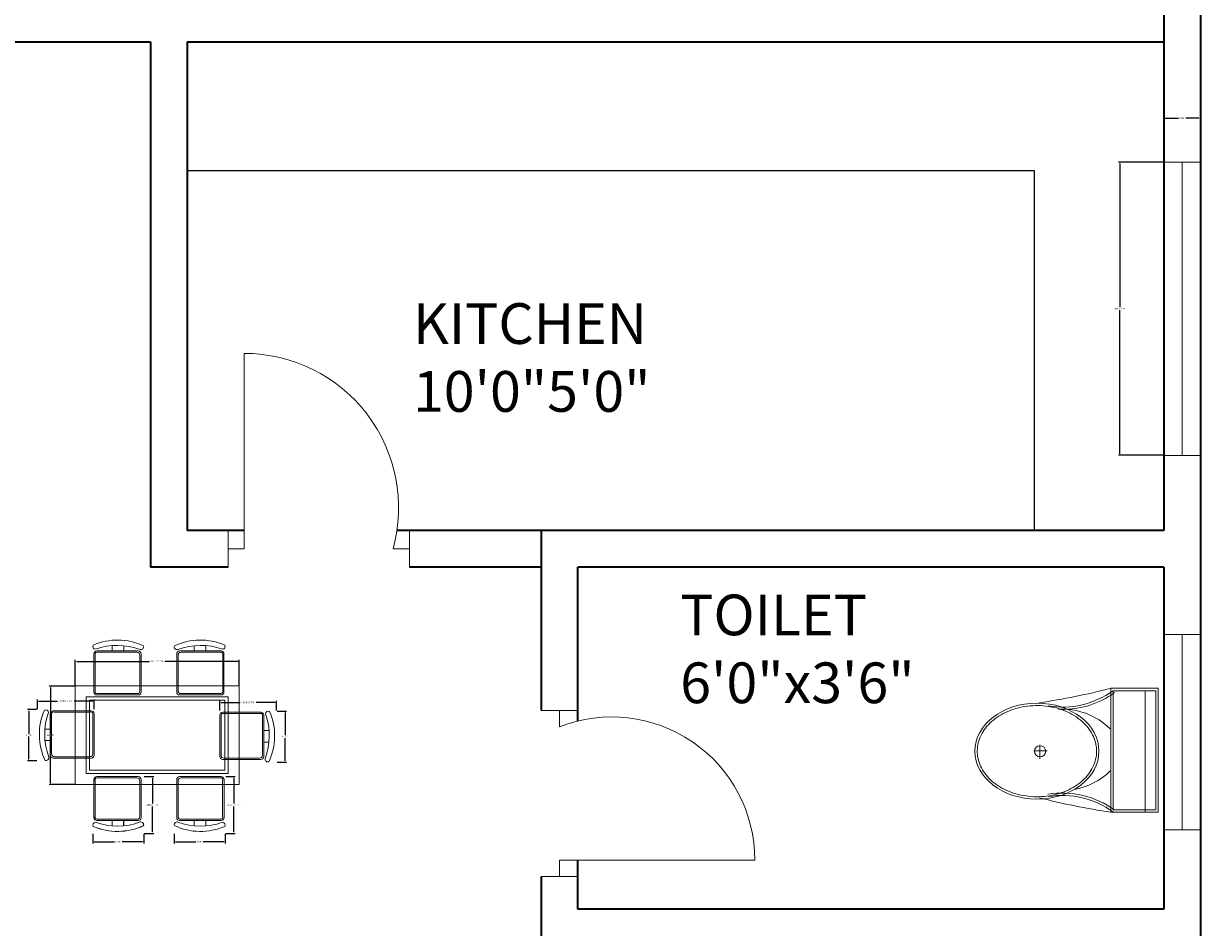
# Model space of a CAD drawing. Units: inches. Extents: x 2234 to 3001, y 1541 to 2386.
# Tile 9 of 12: x 2744 to 2888, y 1891 to 2002. Entities that reach past the tile are written whole.
import ezdxf

# ---------------------------------------------------------------- set-up
doc = ezdxf.new("R2010")
doc.units = ezdxf.units.IN
for name, color, linetype, lineweight in [('A-ANNO-DIMS', 2, 'Continuous', 18), ('A-AREA-IDEN', 7, 'Continuous', 18), ('A-DOOR', 3, 'Continuous', 18), ('A-FLOR-CASE', 8, 'Continuous', 25), ('A-FLOR-FIXT', 9, 'Continuous', 18), ('A-FURN', 9, 'Continuous', 13), ('A-GLAZ', 4, 'Continuous', 18), ('A-WALL', 7, 'Continuous', 35)]:
    doc.layers.add(name, color=color, linetype=linetype, lineweight=lineweight)
doc.styles.get("Standard").update_dxf_attribs({"font": 'arial.ttf'})
doc.dimstyles.get("Standard").update_dxf_attribs({"dimtxt": 0.18, "dimasz": 0.18, "dimexe": 0.18, "dimexo": 0.0625, "dimgap": 0.09, "dimtad": 0, "dimtih": 1, "dimtoh": 1, "dimdec": 4, "dimzin": 0, "dimdsep": 46, "dimtxsty": 'Standard', "dimcen": 0.09, "dimadec": 0, "dimazin": 0, "dimtfac": 1, "dimtdec": 4, "dimtofl": 0, "dimtmove": 0, "dimatfit": 3, "dimfxl": 1, "dimtolj": 1, "dimtzin": 0, "dimarcsym": 0})

# ---------------------------------------------------------------- blocks, each defined once
blk = doc.blocks.new('A$C31115884')
for p, q in [((283.1, 497.7), (223.4, 497.7)), ((257.5, 466.4), (257.5, 523.2)), ((0, 200), (0, 0)), ((520, 200), (0, 200)), ((520, 0), (520, 200)), ((10, 190), (10, 10)), ((510, 190), (10, 190)), ((510, 10), (510, 190)), ((510, 54.5), (0, 54.5)), ((10, 10), (510, 10)), ((0, 0), (520, 0))]:
    blk.add_line(p, q)
blk.add_circle((255.6, 496.4), 23.6)
for centre, radius, start, end in [((2777.7, -204.6), 2807, 165.4549, 171.7133), ((3237, 905), 2807, 188.2867, 194.5451), ((-294.5, 403.3), 364.7, 324.2091, 9.3499), ((-294.5, 403.3), 374.7, 324.2091, 9.3499), ((805.8, 403.3), 364.7, 170.6501, 215.7909), ((139.5, 406.2), 293.5, 315.8436, 2.6563), ((805.8, 403.3), 374.7, 179.2036, 215.7909), ((383.6, 406.2), 293.5, 190.2774, 224.1564)]:
    blk.add_arc(centre, radius, start, end)
blk.add_ellipse((256.2, 509.9), major_axis=(0, -260.7), ratio=0.772727)
blk.add_open_spline([(256.2, 259.2), (263.1, 259.2), (270, 259.7), (287.8, 262.3), (298.7, 265.1), (319.9, 273.1), (330.2, 278.4), (350.1, 291.1), (359.7, 298.7), (377.7, 315.9), (386.2, 325.5), (401.7, 346.6), (408.8, 358.1), (421.3, 382.5), (426.8, 395.5), (435.9, 422.4), (439.5, 436.4), (444.8, 465.1), (446.5, 479.7), (447.9, 509.2), (447.6, 524), (445, 553.3), (442.7, 567.8), (436.3, 596), (432.1, 609.7), (421.9, 636), (416, 648.6), (402.5, 672.1), (395, 683), (378.6, 703), (369.8, 712.1), (351.1, 728), (341.3, 734.8), (320.9, 746.2), (310.4, 750.7), (288.9, 757.3), (278, 759.4), (256, 761), (245, 760.6), (223.1, 757.2), (212.3, 754.3), (191.1, 746.1), (180.8, 740.7), (160.9, 727.8), (151.4, 720.1), (133.5, 702.7), (125.1, 693), (109.6, 671.7), (102.6, 660.2), (90.2, 635.7), (84.9, 622.7), (76, 595.6), (72.4, 581.6), (67.2, 552.9), (65.6, 538.2), (64.4, 508.8), (64.8, 494), (67.5, 464.7), (69.9, 450.2), (76.6, 422), (80.8, 408.3), (91.1, 382.2), (97.2, 369.7), (110.8, 346.3), (118.4, 335.4), (134.8, 315.6), (143.7, 306.7), (162.4, 290.9), (172.3, 284.2), (192.8, 273), (203.3, 268.6), (224.8, 262.2), (235.8, 260.2), (249.9, 259.3), (253, 259.2), (256.2, 259.2)], degree=3, knots=[0, 0, 0, 0, 0.110105, 0.110105, 0.285049, 0.285049, 0.459994, 0.459994, 0.634938, 0.634938, 0.809882, 0.809882, 0.984827, 0.984827, 1.159771, 1.159771, 1.334715, 1.334715, 1.50966, 1.50966, 1.684604, 1.684604, 1.859549, 1.859549, 2.034493, 2.034493, 2.209437, 2.209437, 2.384382, 2.384382, 2.559326, 2.559326, 2.73427, 2.73427, 2.909215, 2.909215, 3.084159, 3.084159, 3.259103, 3.259103, 3.434048, 3.434048, 3.608992, 3.608992, 3.783936, 3.783936, 3.958881, 3.958881, 4.133825, 4.133825, 4.30877, 4.30877, 4.483714, 4.483714, 4.658658, 4.658658, 4.833603, 4.833603, 5.008547, 5.008547, 5.183491, 5.183491, 5.358436, 5.358436, 5.53338, 5.53338, 5.708324, 5.708324, 5.883269, 5.883269, 6.058213, 6.058213, 6.233158, 6.233158, 6.283185, 6.283185, 6.283185, 6.283185])
blk = doc.blocks.new('TABLE-DINING-RECT')
for points in [[(0, 12.09), (20.14, 12.09), (20.14, 0), (0, 0)], [(0, 12.09), (20.14, 12.09), (20.14, 0), (0, 0)], [(1.34, 10.74), (18.8, 10.74), (18.8, 1.34), (1.34, 1.34)], [(1.34, 10.74), (18.8, 10.74), (18.8, 1.34), (1.34, 1.34)], [(1.75, 10.34), (18.4, 10.34), (18.4, 1.75), (1.75, 1.75)], [(1.75, 10.34), (18.4, 10.34), (18.4, 1.75), (1.75, 1.75)]]:
    blk.add_lwpolyline(points, close=True)
blk = doc.blocks.new('CHAIR-DINING-A')
for points in [[(5.76, 1.34, 0.414214), (6.12, 1.7), (6.12, 6.38, 0.414214), (5.76, 6.74), (0.67, 6.74, 0.414214), (0.31, 6.38), (0.31, 1.7, 0.414214), (0.67, 1.34), (5.76, 1.34)], [(5.76, 1.34, 0.414214), (6.12, 1.7), (6.12, 6.38, 0.414214), (5.76, 6.74), (0.67, 6.74, 0.414214), (0.31, 6.38), (0.31, 1.7, 0.414214), (0.67, 1.34), (5.76, 1.34)], [(5.92, 1.12, -0.175809), (0.43, 1.16, 0.578392), (0.02, 0.71, 0.214524), (6.21, 0.62, 0.552014), (5.92, 1.12, -0.065079)], [(5.92, 1.12, -0.175809), (0.43, 1.16, 0.578392), (0.02, 0.71, 0.214524), (6.21, 0.62, 0.552014), (5.92, 1.12, -0.065079)], [(2.45, 1.34), (2.45, 0.7, -0.064759)], [(2.45, 1.34), (2.45, 0.7, -0.064759)]]:
    blk.add_lwpolyline(points, format="xyb")
blk.add_lwpolyline([(5.76, 1.5), (0.83, 1.5, -0.414214), (0.47, 1.86), (0.47, 6.22, -0.414214), (0.83, 6.58), (5.76, 6.58, -0.512069), (5.95, 6.22), (5.95, 1.86, -0.512069)], format="xyb", close=True)
blk.add_lwpolyline([(5.76, 1.5), (0.83, 1.5, -0.414214), (0.47, 1.86), (0.47, 6.22, -0.414214), (0.83, 6.58), (5.76, 6.58, -0.512069), (5.95, 6.22), (5.95, 1.86, -0.512069)], format="xyb", close=True)
blk.add_lwpolyline([(3.88, 0.69), (3.88, 1.34)])
blk.add_lwpolyline([(3.88, 0.69), (3.88, 1.34)])
blk = doc.blocks.new('CHAIR-DINING-B')
for points in [[(5.76, 1.34, 0.414214), (6.12, 1.7), (6.12, 6.38, 0.414214), (5.76, 6.74), (0.67, 6.74, 0.414214), (0.31, 6.38), (0.31, 1.7, 0.414214), (0.67, 1.34), (5.76, 1.34)], [(5.76, 1.34, 0.414214), (6.12, 1.7), (6.12, 6.38, 0.414214), (5.76, 6.74), (0.67, 6.74, 0.414214), (0.31, 6.38), (0.31, 1.7, 0.414214), (0.67, 1.34), (5.76, 1.34)], [(5.92, 1.12, -0.175809), (0.43, 1.16, 0.578392), (0.02, 0.71, 0.214524), (6.21, 0.62, 0.552014), (5.92, 1.12, -0.065079)], [(5.92, 1.12, -0.175809), (0.43, 1.16, 0.578392), (0.02, 0.71, 0.214524), (6.21, 0.62, 0.552014), (5.92, 1.12, -0.065079)], [(2.45, 1.34), (2.45, 0.7, -0.064759)], [(2.45, 1.34), (2.45, 0.7, -0.064759)]]:
    blk.add_lwpolyline(points, format="xyb")
blk.add_lwpolyline([(5.76, 1.5), (0.83, 1.5, -0.414214), (0.47, 1.86), (0.47, 6.22, -0.414214), (0.83, 6.58), (5.76, 6.58, -0.512069), (5.95, 6.22), (5.95, 1.86, -0.512069)], format="xyb", close=True)
blk.add_lwpolyline([(5.76, 1.5), (0.83, 1.5, -0.414214), (0.47, 1.86), (0.47, 6.22, -0.414214), (0.83, 6.58), (5.76, 6.58, -0.512069), (5.95, 6.22), (5.95, 1.86, -0.512069)], format="xyb", close=True)
blk.add_lwpolyline([(3.88, 0.69), (3.88, 1.34)])
blk.add_lwpolyline([(3.88, 0.69), (3.88, 1.34)])
blk = doc.blocks.new('CHAIR-DINING-C')
for points in [[(1.16, 0.43, -0.578392), (0.71, 0.02, -0.214524), (0.62, 6.21, -0.552014), (1.12, 5.92, 0.175809), (1.16, 0.43)], [(1.34, 5.76, -0.414214), (1.7, 6.11), (6.38, 6.11, -0.414214), (6.74, 5.76), (6.74, 0.66, -0.414214), (6.38, 0.31), (1.7, 0.31, -0.414214), (1.34, 0.66), (1.34, 5.76)], [(1.34, 2.45), (0.7, 2.45, 0.064759)]]:
    blk.add_lwpolyline(points, format="xyb")
blk.add_lwpolyline([(1.5, 5.76), (1.5, 0.83, 0.414214), (1.86, 0.47), (6.22, 0.47, 0.414214), (6.58, 0.83), (6.58, 5.76, 0.512069), (6.22, 5.95), (1.86, 5.95, 0.512069)], format="xyb", close=True)
blk.add_lwpolyline([(0.69, 3.88), (1.34, 3.88)])
blk = doc.blocks.new('CHAIR-DINING-F')
for points in [[(5.58, 1.34), (0.49, 1.34, -0.414214), (0.13, 1.7), (0.13, 6.38, -0.414214), (0.49, 6.74), (5.58, 6.74, -0.414214), (5.94, 6.38), (5.94, 1.7, -0.414214), (5.58, 1.34)], [(5.82, 1.16, -0.578392), (6.23, 0.71, -0.214524), (0.04, 0.62, -0.552014), (0.33, 1.12, 0.175809), (5.82, 1.16)], [(3.79, 1.34), (3.79, 0.7, 0.064759)]]:
    blk.add_lwpolyline(points, format="xyb")
blk.add_lwpolyline([(0.49, 1.5), (5.42, 1.5, 0.414214), (5.78, 1.86), (5.78, 6.22, 0.414214), (5.42, 6.58), (0.49, 6.58, 0.512069), (0.29, 6.22), (0.29, 1.86, 0.512069)], format="xyb", close=True)
blk.add_lwpolyline([(2.37, 0.69), (2.37, 1.34)])
blk = doc.blocks.new('WIN-24-A')
for p, q in [((0, 24), (4.5, 24)), ((4.5, 24), (2.25, 24)), ((2.25, 24), (2.25, 0)), ((2.25, 0), (0, 0)), ((0, 0), (4.5, 0))]:
    blk.add_line(p, q)
blk = doc.blocks.new('WIN-36')
for p, q in [((0, 36), (4.5, 36)), ((4.5, 36), (2.25, 36)), ((2.25, 36), (2.25, 0)), ((2.25, 0), (0, 0)), ((0, 0), (4.5, 0))]:
    blk.add_line(p, q)
blk = doc.blocks.new('*D33')
at = {"layer": 'A-ANNO-DIMS', "color": 0, "lineweight": -2, "transparency": 16777216}
for p, q in [((2883.69, 1985.34), (2878.17, 1985.34)), ((2878.35, 1985.16), (2878.35, 1967.52)), ((2878.35, 1949.52), (2878.35, 1967.15)), ((2883.69, 1949.34), (2878.17, 1949.34))]:
    blk.add_line(p, q, dxfattribs=at)
at = {"layer": 'A-ANNO-DIMS', "color": 0, "transparency": 16777216}
for points in [[(2878.32, 1985.16), (2878.38, 1985.16), (2878.35, 1985.34)], [(2878.32, 1949.52), (2878.38, 1949.52), (2878.35, 1949.34)]]:
    blk.add_solid(points, dxfattribs=at)
at = {"layer": 'Defpoints', "color": 0, "transparency": 16777216}
for p in [(2883.75, 1985.34), (2878.35, 1949.34), (2883.75, 1949.34)]:
    blk.add_point(p, dxfattribs=at)
at = {"layer": 'A-ANNO-DIMS', "color": 0, "transparency": 16777216, "insert": (2878.35, 1967.34), "char_height": 0.18, "attachment_point": 5}
blk.add_mtext('\\A1;WIN 36 TYP.', dxfattribs=at)
blk = doc.blocks.new('*D34')
at = {"layer": 'A-ANNO-DIMS', "color": 0, "lineweight": -2, "transparency": 16777216}
for p, q in [((2883.75, 1985.4), (2883.75, 1990.92)), ((2883.93, 1990.74), (2885.55, 1990.74)), ((2888.07, 1990.74), (2886.46, 1990.74)), ((2888.25, 1985.4), (2888.25, 1990.92))]:
    blk.add_line(p, q, dxfattribs=at)
at = {"layer": 'A-ANNO-DIMS', "color": 0, "transparency": 16777216}
for points in [[(2883.93, 1990.77), (2883.93, 1990.71), (2883.75, 1990.74)], [(2888.07, 1990.77), (2888.07, 1990.71), (2888.25, 1990.74)]]:
    blk.add_solid(points, dxfattribs=at)
at = {"layer": 'Defpoints', "color": 0, "transparency": 16777216}
for p in [(2883.75, 1990.74), (2883.75, 1985.34), (2888.25, 1985.34)]:
    blk.add_point(p, dxfattribs=at)
at = {"layer": 'A-ANNO-DIMS', "color": 0, "transparency": 16777216, "insert": (2886, 1990.74), "char_height": 0.18, "attachment_point": 5}
blk.add_mtext('\\A1;5 TYP.', dxfattribs=at)
blk = doc.blocks.new('*D39')
at = {"layer": 'A-ANNO-DIMS', "color": 0, "lineweight": -2, "transparency": 16777216}
for p, q in [((2749.99, 1921.07), (2749.99, 1924.21)), ((2750.17, 1924.03), (2759.1, 1924.03)), ((2769.95, 1924.03), (2761.02, 1924.03)), ((2770.13, 1921.07), (2770.13, 1924.21))]:
    blk.add_line(p, q, dxfattribs=at)
at = {"layer": 'A-ANNO-DIMS', "color": 0, "transparency": 16777216}
for points in [[(2750.17, 1924.06), (2750.17, 1924), (2749.99, 1924.03)], [(2769.95, 1924.06), (2769.95, 1924), (2770.13, 1924.03)]]:
    blk.add_solid(points, dxfattribs=at)
at = {"layer": 'Defpoints', "color": 0, "transparency": 16777216}
for p in [(2770.13, 1924.03), (2749.99, 1921.01), (2770.13, 1921.01)]:
    blk.add_point(p, dxfattribs=at)
at = {"layer": 'A-ANNO-DIMS', "color": 0, "transparency": 16777216, "insert": (2760.06, 1924.03), "char_height": 0.18, "attachment_point": 5}
blk.add_mtext('\\A1;TABLE 20 TYP.', dxfattribs=at)
blk = doc.blocks.new('*D40')
at = {"layer": 'A-ANNO-DIMS', "color": 0, "lineweight": -2, "transparency": 16777216}
for p, q in [((2749.93, 1921.01), (2746.79, 1921.01)), ((2746.97, 1920.83), (2746.97, 1915.15)), ((2746.97, 1909.1), (2746.97, 1914.79)), ((2749.93, 1908.92), (2746.79, 1908.92))]:
    blk.add_line(p, q, dxfattribs=at)
at = {"layer": 'A-ANNO-DIMS', "color": 0, "transparency": 16777216}
for points in [[(2746.94, 1920.83), (2747, 1920.83), (2746.97, 1921.01)], [(2746.94, 1909.1), (2747, 1909.1), (2746.97, 1908.92)]]:
    blk.add_solid(points, dxfattribs=at)
at = {"layer": 'Defpoints', "color": 0, "transparency": 16777216}
for p in [(2746.97, 1921.01), (2749.99, 1921.01), (2749.99, 1908.92)]:
    blk.add_point(p, dxfattribs=at)
at = {"layer": 'A-ANNO-DIMS', "color": 0, "transparency": 16777216, "insert": (2746.97, 1914.97), "char_height": 0.18, "attachment_point": 5}
blk.add_mtext('\\A1;12 TYP.', dxfattribs=at)
blk = doc.blocks.new('*D41')
at = {"layer": 'A-ANNO-DIMS', "color": 0, "lineweight": -2, "transparency": 16777216}
for p, q in [((2767.75, 1918), (2767.75, 1919.17)), ((2774.73, 1918), (2774.73, 1919.17)), ((2767.93, 1918.99), (2770.24, 1918.99)), ((2774.55, 1918.99), (2772.24, 1918.99))]:
    blk.add_line(p, q, dxfattribs=at)
at = {"layer": 'A-ANNO-DIMS', "color": 0, "transparency": 16777216}
for points in [[(2767.93, 1919.02), (2767.93, 1918.96), (2767.75, 1918.99)], [(2774.55, 1919.02), (2774.55, 1918.96), (2774.73, 1918.99)]]:
    blk.add_solid(points, dxfattribs=at)
at = {"layer": 'Defpoints', "color": 0, "transparency": 16777216}
for p in [(2767.75, 1918.99), (2767.75, 1917.94), (2774.73, 1917.94)]:
    blk.add_point(p, dxfattribs=at)
at = {"layer": 'A-ANNO-DIMS', "color": 0, "transparency": 16777216, "insert": (2771.24, 1918.99), "char_height": 0.18, "attachment_point": 5}
blk.add_mtext('\\A1;CHAIR A 7 TYP.', dxfattribs=at)
blk = doc.blocks.new('*D42')
at = {"layer": 'A-ANNO-DIMS', "color": 0, "lineweight": -2, "transparency": 16777216}
for p, q in [((2774.79, 1917.94), (2775.95, 1917.94)), ((2775.77, 1917.76), (2775.77, 1914.98)), ((2775.77, 1911.83), (2775.77, 1914.61)), ((2774.79, 1911.65), (2775.95, 1911.65))]:
    blk.add_line(p, q, dxfattribs=at)
at = {"layer": 'A-ANNO-DIMS', "color": 0, "transparency": 16777216}
for points in [[(2775.74, 1917.76), (2775.8, 1917.76), (2775.77, 1917.94)], [(2775.74, 1911.83), (2775.8, 1911.83), (2775.77, 1911.65)]]:
    blk.add_solid(points, dxfattribs=at)
at = {"layer": 'Defpoints', "color": 0, "transparency": 16777216}
for p in [(2774.73, 1917.94), (2775.77, 1917.94), (2774.73, 1911.65)]:
    blk.add_point(p, dxfattribs=at)
at = {"layer": 'A-ANNO-DIMS', "color": 0, "transparency": 16777216, "insert": (2775.77, 1914.8), "char_height": 0.18, "attachment_point": 5}
blk.add_mtext('\\A1;6 TYP.', dxfattribs=at)
blk = doc.blocks.new('*D43')
at = {"layer": 'A-ANNO-DIMS', "color": 0, "lineweight": -2, "transparency": 16777216}
for p, q in [((2768.48, 1909.89), (2769.64, 1909.89)), ((2769.46, 1909.71), (2769.46, 1906.58)), ((2769.46, 1903.09), (2769.46, 1906.22)), ((2768.48, 1902.91), (2769.64, 1902.91))]:
    blk.add_line(p, q, dxfattribs=at)
at = {"layer": 'A-ANNO-DIMS', "color": 0, "transparency": 16777216}
for points in [[(2769.43, 1909.71), (2769.49, 1909.71), (2769.46, 1909.89)], [(2769.43, 1903.09), (2769.49, 1903.09), (2769.46, 1902.91)]]:
    blk.add_solid(points, dxfattribs=at)
at = {"layer": 'Defpoints', "color": 0, "transparency": 16777216}
for p in [(2768.42, 1909.89), (2769.46, 1909.89), (2768.42, 1902.91)]:
    blk.add_point(p, dxfattribs=at)
at = {"layer": 'A-ANNO-DIMS', "color": 0, "transparency": 16777216, "insert": (2769.46, 1906.4), "char_height": 0.18, "attachment_point": 5}
blk.add_mtext('\\A1;CHAIR B 7 TYP.', dxfattribs=at)
blk = doc.blocks.new('*D44')
at = {"layer": 'A-ANNO-DIMS', "color": 0, "lineweight": -2, "transparency": 16777216}
for p, q in [((2762.13, 1902.85), (2762.13, 1901.69)), ((2762.31, 1901.87), (2764.82, 1901.87)), ((2768.24, 1901.87), (2765.73, 1901.87)), ((2768.42, 1902.85), (2768.42, 1901.69))]:
    blk.add_line(p, q, dxfattribs=at)
at = {"layer": 'A-ANNO-DIMS', "color": 0, "transparency": 16777216}
for points in [[(2762.31, 1901.9), (2762.31, 1901.84), (2762.13, 1901.87)], [(2768.24, 1901.9), (2768.24, 1901.84), (2768.42, 1901.87)]]:
    blk.add_solid(points, dxfattribs=at)
at = {"layer": 'Defpoints', "color": 0, "transparency": 16777216}
for p in [(2762.13, 1902.91), (2768.42, 1902.91), (2768.42, 1901.87)]:
    blk.add_point(p, dxfattribs=at)
at = {"layer": 'A-ANNO-DIMS', "color": 0, "transparency": 16777216, "insert": (2765.27, 1901.87), "char_height": 0.18, "attachment_point": 5}
blk.add_mtext('\\A1;6 TYP.', dxfattribs=at)
blk = doc.blocks.new('*D45')
at = {"layer": 'A-ANNO-DIMS', "color": 0, "lineweight": -2, "transparency": 16777216}
for p, q in [((2745.34, 1918.18), (2745.34, 1919.34)), ((2745.52, 1919.16), (2747.82, 1919.16)), ((2752.14, 1919.16), (2749.84, 1919.16)), ((2752.32, 1918.18), (2752.32, 1919.34))]:
    blk.add_line(p, q, dxfattribs=at)
at = {"layer": 'A-ANNO-DIMS', "color": 0, "transparency": 16777216}
for points in [[(2745.52, 1919.19), (2745.52, 1919.13), (2745.34, 1919.16)], [(2752.14, 1919.19), (2752.14, 1919.13), (2752.32, 1919.16)]]:
    blk.add_solid(points, dxfattribs=at)
at = {"layer": 'Defpoints', "color": 0, "transparency": 16777216}
for p in [(2752.32, 1919.16), (2745.34, 1918.11), (2752.32, 1918.11)]:
    blk.add_point(p, dxfattribs=at)
at = {"layer": 'A-ANNO-DIMS', "color": 0, "transparency": 16777216, "insert": (2748.83, 1919.16), "char_height": 0.18, "attachment_point": 5}
blk.add_mtext('\\A1;CHAIR C 7 TYP.', dxfattribs=at)
blk = doc.blocks.new('*D46')
at = {"layer": 'A-ANNO-DIMS', "color": 0, "lineweight": -2, "transparency": 16777216}
for p, q in [((2745.28, 1918.11), (2744.12, 1918.11)), ((2744.3, 1917.93), (2744.3, 1915.15)), ((2744.3, 1912.01), (2744.3, 1914.79)), ((2745.28, 1911.83), (2744.12, 1911.83))]:
    blk.add_line(p, q, dxfattribs=at)
at = {"layer": 'A-ANNO-DIMS', "color": 0, "transparency": 16777216}
for points in [[(2744.27, 1917.93), (2744.33, 1917.93), (2744.3, 1918.11)], [(2744.27, 1912.01), (2744.33, 1912.01), (2744.3, 1911.83)]]:
    blk.add_solid(points, dxfattribs=at)
at = {"layer": 'Defpoints', "color": 0, "transparency": 16777216}
for p in [(2744.3, 1918.11), (2745.34, 1918.11), (2745.34, 1911.83)]:
    blk.add_point(p, dxfattribs=at)
at = {"layer": 'A-ANNO-DIMS', "color": 0, "transparency": 16777216, "insert": (2744.3, 1914.97), "char_height": 0.18, "attachment_point": 5}
blk.add_mtext('\\A1;6 TYP.', dxfattribs=at)
blk = doc.blocks.new('*D51')
at = {"layer": 'A-ANNO-DIMS', "color": 0, "lineweight": -2, "transparency": 16777216}
for p, q in [((2758.48, 1909.89), (2759.65, 1909.89)), ((2759.47, 1909.71), (2759.47, 1906.58)), ((2759.47, 1903.09), (2759.47, 1906.22)), ((2758.48, 1902.91), (2759.65, 1902.91))]:
    blk.add_line(p, q, dxfattribs=at)
at = {"layer": 'A-ANNO-DIMS', "color": 0, "transparency": 16777216}
for points in [[(2759.44, 1909.71), (2759.5, 1909.71), (2759.47, 1909.89)], [(2759.44, 1903.09), (2759.5, 1903.09), (2759.47, 1902.91)]]:
    blk.add_solid(points, dxfattribs=at)
at = {"layer": 'Defpoints', "color": 0, "transparency": 16777216}
for p in [(2758.42, 1909.89), (2759.47, 1909.89), (2758.42, 1902.91)]:
    blk.add_point(p, dxfattribs=at)
at = {"layer": 'A-ANNO-DIMS', "color": 0, "transparency": 16777216, "insert": (2759.47, 1906.4), "char_height": 0.18, "attachment_point": 5}
blk.add_mtext('\\A1;CHAIR F 7 TYP.', dxfattribs=at)
blk = doc.blocks.new('*D52')
at = {"layer": 'A-ANNO-DIMS', "color": 0, "lineweight": -2, "transparency": 16777216}
for p, q in [((2752.14, 1902.85), (2752.14, 1901.69)), ((2752.32, 1901.87), (2754.82, 1901.87)), ((2758.24, 1901.87), (2755.74, 1901.87)), ((2758.42, 1902.85), (2758.42, 1901.69))]:
    blk.add_line(p, q, dxfattribs=at)
at = {"layer": 'A-ANNO-DIMS', "color": 0, "transparency": 16777216}
for points in [[(2752.32, 1901.9), (2752.32, 1901.84), (2752.14, 1901.87)], [(2758.24, 1901.9), (2758.24, 1901.84), (2758.42, 1901.87)]]:
    blk.add_solid(points, dxfattribs=at)
at = {"layer": 'Defpoints', "color": 0, "transparency": 16777216}
for p in [(2752.14, 1902.91), (2758.42, 1902.91), (2758.42, 1901.87)]:
    blk.add_point(p, dxfattribs=at)
at = {"layer": 'A-ANNO-DIMS', "color": 0, "transparency": 16777216, "insert": (2755.28, 1901.87), "char_height": 0.18, "attachment_point": 5}
blk.add_mtext('\\A1;6 TYP.', dxfattribs=at)

msp = doc.modelspace()

# ---------------------------------------------------------------- linework, layer by layer
at = {"layer": 'A-DOOR'}
for p, q in [((2770.7619, 1937.861), (2770.7619, 1961.861)), ((2768.7619, 1940.111), (2768.7619, 1935.611)), ((2791.045, 1940.111), (2791.045, 1935.611)), ((2768.7619, 1935.611), (2768.7619, 1937.861)), ((2768.7619, 1937.861), (2770.7619, 1937.861)), ((2791.045, 1937.861), (2789.045, 1937.861)), ((2791.045, 1935.611), (2791.045, 1937.861)), ((2807.2534, 1917.9944), (2811.7534, 1917.9944)), ((2811.7534, 1917.9944), (2809.5034, 1917.9944)), ((2809.5034, 1917.9944), (2809.5034, 1915.9944)), ((2809.5034, 1897.6296), (2809.5034, 1899.6296)), ((2809.5034, 1899.6296), (2833.5034, 1899.6296)), ((2811.7534, 1897.6296), (2807.2534, 1897.6296)), ((2807.2534, 1897.6296), (2809.5034, 1897.6296))]:
    msp.add_line(p, q, dxfattribs=at)
for centre, radius, start, end in [((2770.7619, 1942.897), 18.9641, 344.600238, 90), ((2815.9241, 1899.6296), 17.5793, 0, 111.422342)]:
    msp.add_arc(centre, radius, start, end, dxfattribs=at)
at = {"layer": 'A-FLOR-CASE'}
for p, q in [((2763.7534, 1984.3319), (2867.8031, 1984.3319)), ((2867.8031, 1984.3319), (2867.8031, 1940.111))]:
    msp.add_line(p, q, dxfattribs=at)
at = {"layer": 'A-FURN'}
for points in [[(2752.4807, 1925.5315, -0.17580919), (2757.9674, 1925.4899, 0.57839206), (2758.383, 1925.947, 0.21452438), (2752.1898, 1926.0301, 0.55201397), (2752.4807, 1925.5315, -0.06507904)], [(2752.4808, 1925.5312, -0.17580919), (2757.9674, 1925.4897, 0.57839206), (2758.383, 1925.9467, 0.21452438), (2752.1898, 1926.0298, 0.55201397), (2752.4808, 1925.5312, -0.06507904)], [(2762.5864, 1925.4899, -0.57839206), (2762.1708, 1925.947, -0.21452438), (2768.364, 1926.0301, -0.55201397), (2768.0731, 1925.5315, 0.1758092), (2762.5864, 1925.4899)], [(2762.5864, 1925.4897, -0.57839206), (2762.1708, 1925.9467, -0.21452438), (2768.364, 1926.0298, -0.55201397), (2768.0731, 1925.5312, 0.1758092), (2762.5864, 1925.4897)], [(2757.7346, 1925.3113), (2752.641, 1925.3113, 0.41421356), (2752.2846, 1924.9549), (2752.2846, 1920.2714, 0.41421356), (2752.641, 1919.9151), (2757.7346, 1919.9151, 0.41421356), (2758.091, 1920.2714), (2758.091, 1924.9549, 0.41421356), (2757.7346, 1925.3113)], [(2757.7346, 1925.311), (2752.641, 1925.311, 0.41421356), (2752.2847, 1924.9547), (2752.2847, 1920.2712, 0.41421356), (2752.641, 1919.9149), (2757.7346, 1919.9149, 0.41421356), (2758.091, 1920.2712), (2758.091, 1924.9547, 0.41421356), (2757.7346, 1925.311)], [(2755.9455, 1925.3113), (2755.9455, 1925.9554, -0.06475861)], [(2755.9455, 1925.311), (2755.9455, 1925.9552, -0.06475861)], [(2767.9128, 1925.3113, -0.41421356), (2768.2692, 1924.9549), (2768.2692, 1920.2714, -0.41421356), (2767.9128, 1919.9151), (2762.8192, 1919.9151, -0.41421356), (2762.4628, 1920.2714), (2762.4628, 1924.9549, -0.41421356), (2762.8192, 1925.3113), (2767.9128, 1925.3113)], [(2767.9128, 1925.311, -0.41421356), (2768.2692, 1924.9547), (2768.2692, 1920.2712, -0.41421356), (2767.9128, 1919.9149), (2762.8192, 1919.9149, -0.41421356), (2762.4629, 1920.2712), (2762.4629, 1924.9547, -0.41421356), (2762.8192, 1925.311), (2767.9128, 1925.311)], [(2764.6083, 1925.3113), (2764.6083, 1925.9554, 0.06475861)], [(2764.6083, 1925.311), (2764.6083, 1925.9552, 0.06475861)], [(2757.7346, 1904.4919), (2752.641, 1904.4919, -0.41421356), (2752.2847, 1904.8482), (2752.2847, 1909.5317, -0.41421356), (2752.641, 1909.888), (2757.7346, 1909.888, -0.41421356), (2758.091, 1909.5317), (2758.091, 1904.8482, -0.41421356), (2757.7346, 1904.4919)], [(2757.9674, 1904.3132, -0.57839206), (2758.383, 1903.8562, -0.21452438), (2752.1898, 1903.7731, -0.55201397), (2752.4808, 1904.2716, 0.17580929), (2757.9674, 1904.3132)], [(2755.9455, 1904.4919), (2755.9455, 1903.8477, 0.06475861)]]:
    msp.add_lwpolyline(points, format="xyb", dxfattribs=at)
for points in [[(2752.6432, 1925.1507), (2757.5741, 1925.1507, -0.41421356), (2757.9304, 1924.7944), (2757.9304, 1920.432, -0.41421356), (2757.5741, 1920.0756), (2752.6432, 1920.0756, -0.51206948), (2752.4452, 1920.432), (2752.4452, 1924.7944, -0.51206948)], [(2752.6432, 1925.1505), (2757.5741, 1925.1505, -0.41421356), (2757.9304, 1924.7941), (2757.9304, 1920.4318, -0.41421356), (2757.5741, 1920.0754), (2752.6432, 1920.0754, -0.51206948), (2752.4452, 1920.4318), (2752.4452, 1924.7941, -0.51206948)], [(2767.9106, 1925.1507), (2762.9797, 1925.1507, 0.41421356), (2762.6234, 1924.7944), (2762.6234, 1920.432, 0.41421356), (2762.9797, 1920.0756), (2767.9106, 1920.0756, 0.51206948), (2768.1086, 1920.432), (2768.1086, 1924.7944, 0.51206948)], [(2767.9107, 1925.1505), (2762.9797, 1925.1505, 0.41421356), (2762.6234, 1924.7941), (2762.6234, 1920.4318, 0.41421356), (2762.9797, 1920.0754), (2767.9107, 1920.0754, 0.51206948), (2768.1086, 1920.4318), (2768.1086, 1924.7941, 0.51206948)], [(2752.6432, 1904.6524), (2757.5741, 1904.6524, 0.41421356), (2757.9304, 1905.0088), (2757.9304, 1909.3711, 0.41421356), (2757.5741, 1909.7275), (2752.6432, 1909.7275, 0.51206948), (2752.4452, 1909.3711), (2752.4452, 1905.0088, 0.51206948)]]:
    msp.add_lwpolyline(points, format="xyb", close=True, dxfattribs=at)
for points in [[(2754.5197, 1925.9671), (2754.5197, 1925.3113)], [(2754.5197, 1925.9669), (2754.5197, 1925.311)], [(2766.0341, 1925.9671), (2766.0341, 1925.3113)], [(2766.0341, 1925.9669), (2766.0341, 1925.311)], [(2754.5197, 1903.836), (2754.5197, 1904.4919)]]:
    msp.add_lwpolyline(points, dxfattribs=at)
at = {"layer": 'A-WALL'}
for p, q in [((2888.2534, 2298.611), (2888.2534, 1702.111)), ((2883.7534, 2064.611), (2883.7534, 1940.111)), ((2642.9141, 2000.111), (2759.2534, 2000.111)), ((2759.2534, 2000.111), (2759.2534, 1935.611)), ((2763.7534, 2000.111), (2883.7534, 2000.111)), ((2763.7534, 2000.111), (2763.7534, 1940.111)), ((2770.7619, 1940.111), (2763.7534, 1940.111)), ((2883.7534, 1940.111), (2789.5202, 1940.111)), ((2807.2534, 1940.111), (2807.2534, 1917.9944)), ((2768.7619, 1935.611), (2759.2534, 1935.611)), ((2807.2534, 1935.611), (2791.045, 1935.611)), ((2883.7534, 1935.611), (2811.7534, 1935.611)), ((2811.7534, 1916.707), (2811.7534, 1935.611)), ((2883.7534, 1935.611), (2883.7534, 1893.611)), ((2811.7534, 1893.611), (2811.7534, 1899.6296)), ((2807.2534, 1897.6296), (2807.2534, 1872.7928)), ((2883.7534, 1893.611), (2811.7534, 1893.611)), ((2883.7534, 1893.611), (2811.7534, 1893.611))]:
    msp.add_line(p, q, dxfattribs=at)

# ---------------------------------------------------------------- block references
at = {"layer": 'A-FLOR-FIXT', "xscale": 0.0292470664339069, "yscale": 0.0292470664339069, "zscale": 0.0292470664339069, "rotation": 89.99999999999999}
msp.add_blockref('A$C31115884', (2883.0713, 1905.5179), dxfattribs=at)
at = {"layer": 'A-FURN'}
for name, p in [('TABLE-DINING-RECT', (2749.9889, 1908.9231)), ('CHAIR-DINING-C', (2745.578, 1911.8502)), ('CHAIR-DINING-C', (2745.578, 1911.85)), ('CHAIR-DINING-F', (2752.151, 1903.151)), ('CHAIR-DINING-B', (2762.154, 1903.15))]:
    msp.add_blockref(name, p, dxfattribs=at)
at = {"layer": 'A-FURN', "rotation": 90}
msp.add_blockref('CHAIR-DINING-A', (2774.4909, 1911.675), dxfattribs=at)
at = {"layer": 'A-GLAZ', "rotation": 180}
for name, p in [('WIN-36', (2888.2539, 1985.3364)), ('WIN-24-A', (2888.2539, 1927.3337))]:
    msp.add_blockref(name, p, dxfattribs=at)

# ---------------------------------------------------------------- texts
at = {"layer": 'A-AREA-IDEN', "char_height": 5, "attachment_point": 1}
for s, width, insert in [('KITCHEN\\P10\'0"5\'0"', 128.41698, (2791.4891, 1968.0203)), ('TOILET\\P6\'0"x3\'6"', 57.235301, (2824.3279, 1932.2383))]:
    msp.add_mtext_dynamic_manual_height_columns(s, width=width, gutter_width=12.5, heights=[0], dxfattribs=dict(at, insert=insert))

# ---------------------------------------------------------------- dimensions: what is measured, and where the dimension line sits
at = {"layer": 'A-ANNO-DIMS'}
for base, p1, p2, angle, text, picture, middle in [((2883.7534479173, 1990.7361552143), (2888.2534479174, 1985.3361552143), (2883.7534479173, 1985.3361552143), 180, '<> TYP.', '*D34', (2886.0034479173, 1990.7361552143)), ((2878.3534, 1949.3362), (2883.7534, 1985.3362), (2883.7534, 1949.3362), 270, 'WIN <> TYP.', '*D33', (2878.3534, 1967.3362)), ((2746.9676, 1921.0096), (2749.9891, 1908.923), (2749.9891, 1921.0096), 90, '<> TYP.', '*D40', (2746.9676, 1914.9663)), ((2767.7527, 1918.9855), (2774.7272, 1917.9393), (2767.7527, 1917.9393), 180, 'CHAIR A <> TYP.', '*D41', (2771.24, 1918.9855)), ((2744.2951, 1918.1136), (2745.3412, 1911.8272), (2745.3412, 1918.1136), 90, '<> TYP.', '*D46', (2744.2951, 1914.9704)), ((2775.7734, 1917.9393), (2774.7272, 1911.6529), (2774.7272, 1917.9393), 90, '<> TYP.', '*D42', (2775.7734, 1914.7961)), ((2759.4682, 1909.8883), (2758.422, 1902.914), (2758.422, 1909.8883), 90, 'CHAIR F <> TYP.', '*D51', (2759.4682, 1906.4011)), ((2769.4644, 1909.8883), (2768.4182, 1902.9137), (2768.4182, 1909.8883), 90, 'CHAIR B <> TYP.', '*D43', (2769.4644, 1906.401))]:
    dim = msp.add_linear_dim(base=base, p1=p1, p2=p2, angle=angle, text=text, dimstyle='Standard', override={"dimdec": 0, "dimlfac": 1, "dimrnd": 0, "dimzin": 0, "dimdsep": 46, "dimlunit": 2}, dxfattribs=at)
    dim.commit()
    dim.dimension.update_dxf_attribs({"geometry": picture, "text_midpoint": middle})
for base, p1, p2, text, picture, middle in [((2770.1331, 1924.0312), (2749.9891, 1921.0096), (2770.1331, 1921.0096), 'TABLE <> TYP.', '*D39', (2760.0611, 1924.0312)), ((2752.3155, 1919.1598), (2745.3412, 1918.1136), (2752.3155, 1918.1136), 'CHAIR C <> TYP.', '*D45', (2748.8284, 1919.1598)), ((2758.422, 1901.8678), (2752.1356, 1902.914), (2758.422, 1902.914), '<> TYP.', '*D52', (2755.2788, 1901.8678)), ((2768.4182, 1901.8676), (2762.1318, 1902.9137), (2768.4182, 1902.9137), '<> TYP.', '*D44', (2765.275, 1901.8676))]:
    dim = msp.add_linear_dim(base=base, p1=p1, p2=p2, text=text, dimstyle='Standard', override={"dimdec": 0, "dimlfac": 1, "dimrnd": 0, "dimzin": 0, "dimdsep": 46, "dimlunit": 2}, dxfattribs=at)
    dim.commit()
    dim.dimension.update_dxf_attribs({"geometry": picture, "text_midpoint": middle})

doc.saveas('drawing.dxf')
